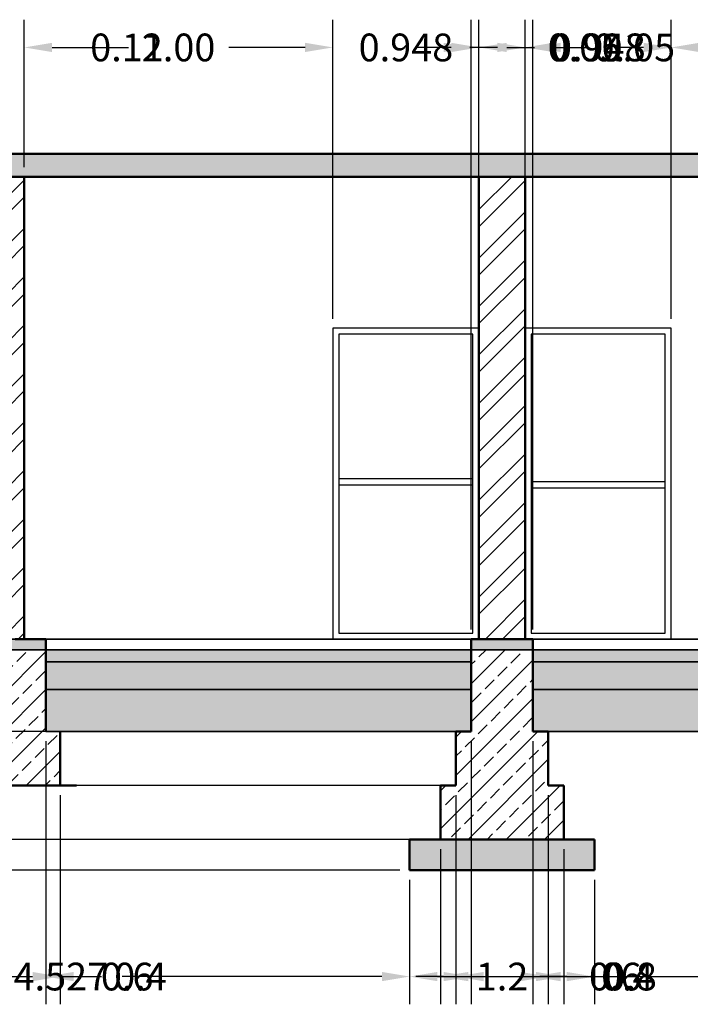
# Model space of a CAD drawing. Units: metres. Extents: x 2294.9 to 2311.3, y 1642.1 to 1648.4.
# Tile 2 of 3: x 2299.8 to 2304.1, y 1642.1 to 1648.4. Entities that reach past the tile are written whole.
import ezdxf

# ---------------------------------------------------------------- set-up
doc = ezdxf.new("R2010")
doc.units = ezdxf.units.M
for name, color, linetype, lineweight in [('A-ANNO-DIMS', 2, 'Continuous', 18), ('A-DOOR', 4, 'Continuous', 25), ('A-FLOR', 3, 'Continuous', 35), ('A-FLOR-PATT', 8, 'Continuous', 13), ('A-WALL', 7, 'Continuous', 50), ('A-WALL-PATT', 8, 'Continuous', 13), ('S-FNDN', 1, 'Continuous', 50), ('S-FNDN-PATT', 8, 'Continuous', 13), ('S-SLAB', 1, 'Continuous', 50), ('S-SLAB-PATT', 8, 'Continuous', 13)]:
    doc.layers.add(name, color=color, linetype=linetype, lineweight=lineweight)
doc.styles.get("Standard").update_dxf_attribs({"font": 'arial.ttf'})
doc.dimstyles.get("Standard").update_dxf_attribs({"dimtxt": 0.18, "dimasz": 0.18, "dimexe": 0.18, "dimexo": 0.0625, "dimgap": 0.09, "dimtad": 0, "dimtih": 1, "dimtoh": 1, "dimdec": 4, "dimzin": 0, "dimdsep": 46, "dimtxsty": 'Standard', "dimcen": 0.09, "dimadec": 0, "dimazin": 0, "dimtfac": 1, "dimtdec": 4, "dimtofl": 0, "dimtmove": 0, "dimatfit": 3, "dimfxl": 1, "dimtolj": 1, "dimtzin": 0, "dimarcsym": 0})

# ---------------------------------------------------------------- blocks, each defined once
blk = doc.blocks.new('FOOTING-PCC-PAD')
for p, q in [((1.1996, 0.1999), (-0.0004, 0.1999)), ((-0.0004, 0.1999), (-0.0004, -0.0001)), ((1.1996, -0.0001), (1.1996, 0.1999)), ((-0.0004, -0.0001), (1.1996, -0.0001))]:
    blk.add_line(p, q)
blk = doc.blocks.new('*D8')
at = {"layer": 'A-ANNO-DIMS', "color": 0, "lineweight": -2, "transparency": 16777216}
for p, q in [((2299.6895, 1647.4894), (2299.6895, 1648.4469)), ((2299.8007, 1647.4894), (2299.8007, 1648.4469)), ((2299.5095, 1648.2669), (2299.3295, 1648.2669)), ((2299.9807, 1648.2669), (2300.1607, 1648.2669))]:
    blk.add_line(p, q, dxfattribs=at)
at = {"layer": 'A-ANNO-DIMS', "color": 0, "transparency": 16777216}
for points in [[(2299.5095, 1648.2969), (2299.5095, 1648.2369), (2299.6895, 1648.2669)], [(2299.9807, 1648.2969), (2299.9807, 1648.2369), (2299.8007, 1648.2669)]]:
    blk.add_solid(points, dxfattribs=at)
at = {"layer": 'Defpoints', "color": 0, "transparency": 16777216}
for p in [(2299.8007, 1648.2669), (2299.6895, 1647.4269), (2299.8007, 1647.4269)]:
    blk.add_point(p, dxfattribs=at)
at = {"layer": 'A-ANNO-DIMS', "color": 0, "transparency": 16777216, "insert": (2300.4671, 1648.2669), "char_height": 0.18, "attachment_point": 5}
blk.add_mtext('\\A1;0.11', dxfattribs=at)
blk = doc.blocks.new('*D9')
at = {"layer": 'A-ANNO-DIMS', "color": 0, "lineweight": -2, "transparency": 16777216}
for p, q in [((2299.8007, 1647.4894), (2299.8007, 1648.4469)), ((2301.8034, 1646.5066), (2301.8034, 1648.4469)), ((2299.9807, 1648.2669), (2300.4771, 1648.2669)), ((2301.6234, 1648.2669), (2301.1271, 1648.2669))]:
    blk.add_line(p, q, dxfattribs=at)
at = {"layer": 'A-ANNO-DIMS', "color": 0, "transparency": 16777216}
for points in [[(2299.9807, 1648.2969), (2299.9807, 1648.2369), (2299.8007, 1648.2669)], [(2301.6234, 1648.2969), (2301.6234, 1648.2369), (2301.8034, 1648.2669)]]:
    blk.add_solid(points, dxfattribs=at)
at = {"layer": 'Defpoints', "color": 0, "transparency": 16777216}
for p in [(2301.8034, 1648.2669), (2299.8007, 1647.4269), (2301.8034, 1646.4441)]:
    blk.add_point(p, dxfattribs=at)
at = {"layer": 'A-ANNO-DIMS', "color": 0, "transparency": 16777216, "insert": (2300.8021, 1648.2669), "char_height": 0.18, "attachment_point": 5}
blk.add_mtext('\\A1;2.00', dxfattribs=at)
blk = doc.blocks.new('*D10')
at = {"layer": 'A-ANNO-DIMS', "color": 0, "lineweight": -2, "transparency": 16777216}
for p, q in [((2301.803421, 1646.506639), (2301.803421, 1648.446914)), ((2302.751389, 1647.489414), (2302.751389, 1648.446914)), ((2301.623421, 1648.266914), (2301.443421, 1648.266914)), ((2302.931389, 1648.266914), (2303.111389, 1648.266914))]:
    blk.add_line(p, q, dxfattribs=at)
at = {"layer": 'A-ANNO-DIMS', "color": 0, "transparency": 16777216}
for points in [[(2301.623421, 1648.296914), (2301.623421, 1648.236914), (2301.803421, 1648.266914)], [(2302.931389, 1648.296914), (2302.931389, 1648.236914), (2302.751389, 1648.266914)]]:
    blk.add_solid(points, dxfattribs=at)
at = {"layer": 'Defpoints', "color": 0, "transparency": 16777216}
for p in [(2302.751389, 1648.266914), (2302.751389, 1647.426914), (2301.803421, 1646.444139)]:
    blk.add_point(p, dxfattribs=at)
at = {"layer": 'A-ANNO-DIMS', "color": 0, "transparency": 16777216, "insert": (2302.277405, 1648.266914), "char_height": 0.18, "attachment_point": 5}
blk.add_mtext('\\A1;0.948', dxfattribs=at)
blk = doc.blocks.new('*D11')
at = {"layer": 'A-ANNO-DIMS', "color": 0, "lineweight": -2, "transparency": 16777216}
for p, q in [((2302.7514, 1647.4894), (2302.7514, 1648.4469)), ((2303.0514, 1647.4894), (2303.0514, 1648.4469)), ((2302.5714, 1648.2669), (2302.3914, 1648.2669)), ((2303.2314, 1648.2669), (2303.4114, 1648.2669))]:
    blk.add_line(p, q, dxfattribs=at)
at = {"layer": 'A-ANNO-DIMS', "color": 0, "transparency": 16777216}
for points in [[(2302.5714, 1648.2969), (2302.5714, 1648.2369), (2302.7514, 1648.2669)], [(2303.2314, 1648.2969), (2303.2314, 1648.2369), (2303.0514, 1648.2669)]]:
    blk.add_solid(points, dxfattribs=at)
at = {"layer": 'Defpoints', "color": 0, "transparency": 16777216}
for p in [(2303.0514, 1648.2669), (2302.7514, 1647.4269), (2303.0514, 1647.4269)]:
    blk.add_point(p, dxfattribs=at)
at = {"layer": 'A-ANNO-DIMS', "color": 0, "transparency": 16777216, "insert": (2303.6652, 1648.2669), "char_height": 0.18, "attachment_point": 5}
blk.add_mtext('\\A1;0.3', dxfattribs=at)
blk = doc.blocks.new('*D12')
at = {"layer": 'A-ANNO-DIMS', "color": 0, "lineweight": -2, "transparency": 16777216}
for p, q in [((2303.0514, 1647.4894), (2303.0514, 1648.4469)), ((2303.9994, 1646.5066), (2303.9994, 1648.4469)), ((2302.8714, 1648.2669), (2302.6914, 1648.2669)), ((2304.1794, 1648.2669), (2304.3594, 1648.2669))]:
    blk.add_line(p, q, dxfattribs=at)
at = {"layer": 'A-ANNO-DIMS', "color": 0, "transparency": 16777216}
for points in [[(2302.8714, 1648.2969), (2302.8714, 1648.2369), (2303.0514, 1648.2669)], [(2304.1794, 1648.2969), (2304.1794, 1648.2369), (2303.9994, 1648.2669)]]:
    blk.add_solid(points, dxfattribs=at)
at = {"layer": 'Defpoints', "color": 0, "transparency": 16777216}
for p in [(2303.9994, 1648.2669), (2303.0514, 1647.4269), (2303.9994, 1646.4441)]:
    blk.add_point(p, dxfattribs=at)
at = {"layer": 'A-ANNO-DIMS', "color": 0, "transparency": 16777216, "insert": (2303.5254, 1648.2669), "char_height": 0.18, "attachment_point": 5}
blk.add_mtext('\\A1;0.948', dxfattribs=at)
blk = doc.blocks.new('*D13')
at = {"layer": 'A-ANNO-DIMS', "color": 0, "lineweight": -2, "transparency": 16777216}
for p, q in [((2303.9994, 1646.5066), (2303.9994, 1648.4469)), ((2304.2214, 1646.5066), (2304.2214, 1648.4469)), ((2303.8194, 1648.2669), (2303.6394, 1648.2669)), ((2304.4014, 1648.2669), (2304.5814, 1648.2669))]:
    blk.add_line(p, q, dxfattribs=at)
at = {"layer": 'A-ANNO-DIMS', "color": 0, "transparency": 16777216}
for points in [[(2303.8194, 1648.2969), (2303.8194, 1648.2369), (2303.9994, 1648.2669)], [(2304.4014, 1648.2969), (2304.4014, 1648.2369), (2304.2214, 1648.2669)]]:
    blk.add_solid(points, dxfattribs=at)
at = {"layer": 'Defpoints', "color": 0, "transparency": 16777216}
for p in [(2304.2214, 1648.2669), (2303.9994, 1646.4441), (2304.2214, 1646.4441)]:
    blk.add_point(p, dxfattribs=at)
at = {"layer": 'A-ANNO-DIMS', "color": 0, "transparency": 16777216, "insert": (2304.9742, 1648.2669), "char_height": 0.18, "attachment_point": 5}
blk.add_mtext('\\A1;0.222', dxfattribs=at)
blk = doc.blocks.new('*D19')
at = {"layer": 'A-ANNO-DIMS', "color": 0, "lineweight": -2, "transparency": 16777216}
for p, q in [((2297.7746, 1642.8644), (2297.7746, 1642.0569)), ((2302.3014, 1642.8644), (2302.3014, 1642.0569)), ((2297.9546, 1642.2369), (2299.6407, 1642.2369)), ((2302.1214, 1642.2369), (2300.4353, 1642.2369))]:
    blk.add_line(p, q, dxfattribs=at)
at = {"layer": 'A-ANNO-DIMS', "color": 0, "transparency": 16777216}
for points in [[(2297.9546, 1642.2669), (2297.9546, 1642.2069), (2297.7746, 1642.2369)], [(2302.1214, 1642.2669), (2302.1214, 1642.2069), (2302.3014, 1642.2369)]]:
    blk.add_solid(points, dxfattribs=at)
at = {"layer": 'Defpoints', "color": 0, "transparency": 16777216}
for p in [(2297.7746, 1642.9269), (2302.3014, 1642.9269), (2302.3014, 1642.2369)]:
    blk.add_point(p, dxfattribs=at)
at = {"layer": 'A-ANNO-DIMS', "color": 0, "transparency": 16777216, "insert": (2300.038, 1642.2369), "char_height": 0.18, "attachment_point": 5}
blk.add_mtext('\\A1;4.527', dxfattribs=at)
blk = doc.blocks.new('*D20')
at = {"layer": 'A-ANNO-DIMS', "color": 0, "lineweight": -2, "transparency": 16777216}
for p, q in [((2302.3014, 1642.8644), (2302.3014, 1642.0569)), ((2303.5014, 1642.8644), (2303.5014, 1642.0569)), ((2302.4814, 1642.2369), (2302.6569, 1642.2369)), ((2303.3214, 1642.2369), (2303.1459, 1642.2369))]:
    blk.add_line(p, q, dxfattribs=at)
at = {"layer": 'A-ANNO-DIMS', "color": 0, "transparency": 16777216}
for points in [[(2302.4814, 1642.2669), (2302.4814, 1642.2069), (2302.3014, 1642.2369)], [(2303.3214, 1642.2669), (2303.3214, 1642.2069), (2303.5014, 1642.2369)]]:
    blk.add_solid(points, dxfattribs=at)
at = {"layer": 'Defpoints', "color": 0, "transparency": 16777216}
for p in [(2302.3014, 1642.9269), (2303.5014, 1642.9269), (2303.5014, 1642.2369)]:
    blk.add_point(p, dxfattribs=at)
at = {"layer": 'A-ANNO-DIMS', "color": 0, "transparency": 16777216, "insert": (2302.9014, 1642.2369), "char_height": 0.18, "attachment_point": 5}
blk.add_mtext('\\A1;1.2', dxfattribs=at)
blk = doc.blocks.new('*D21')
at = {"layer": 'A-ANNO-DIMS', "color": 0, "lineweight": -2, "transparency": 16777216}
for p, q in [((2302.3014, 1642.8644), (2302.3014, 1642.0569)), ((2308.0253, 1642.8644), (2308.0253, 1642.0569)), ((2302.4814, 1642.2369), (2304.77, 1642.2369)), ((2307.8453, 1642.2369), (2305.5567, 1642.2369))]:
    blk.add_line(p, q, dxfattribs=at)
at = {"layer": 'A-ANNO-DIMS', "color": 0, "transparency": 16777216}
for points in [[(2302.4814, 1642.2669), (2302.4814, 1642.2069), (2302.3014, 1642.2369)], [(2307.8453, 1642.2669), (2307.8453, 1642.2069), (2308.0253, 1642.2369)]]:
    blk.add_solid(points, dxfattribs=at)
at = {"layer": 'Defpoints', "color": 0, "transparency": 16777216}
for p in [(2302.3014, 1642.9269), (2308.0253, 1642.9269), (2308.0253, 1642.2369)]:
    blk.add_point(p, dxfattribs=at)
at = {"layer": 'A-ANNO-DIMS', "color": 0, "transparency": 16777216, "insert": (2305.1633, 1642.2369), "char_height": 0.18, "attachment_point": 5}
blk.add_mtext('\\A1;5.724', dxfattribs=at)
blk = doc.blocks.new('*D23')
at = {"layer": 'A-ANNO-DIMS', "color": 0, "lineweight": -2, "transparency": 16777216}
for p, q in [((2299.5412, 1643.7644), (2299.5412, 1642.0569)), ((2299.9412, 1643.7644), (2299.9412, 1642.0569)), ((2299.3612, 1642.2369), (2299.1812, 1642.2369)), ((2300.1212, 1642.2369), (2300.3012, 1642.2369))]:
    blk.add_line(p, q, dxfattribs=at)
at = {"layer": 'A-ANNO-DIMS', "color": 0, "transparency": 16777216}
for points in [[(2299.3612, 1642.2669), (2299.3612, 1642.2069), (2299.5412, 1642.2369)], [(2300.1212, 1642.2669), (2300.1212, 1642.2069), (2299.9412, 1642.2369)]]:
    blk.add_solid(points, dxfattribs=at)
at = {"layer": 'Defpoints', "color": 0, "transparency": 16777216}
for p in [(2299.5412, 1643.8269), (2299.9412, 1643.8269), (2299.9412, 1642.2369)]:
    blk.add_point(p, dxfattribs=at)
at = {"layer": 'A-ANNO-DIMS', "color": 0, "transparency": 16777216, "insert": (2300.5547, 1642.2369), "char_height": 0.18, "attachment_point": 5}
blk.add_mtext('\\A1;0.4', dxfattribs=at)
blk = doc.blocks.new('*D24')
at = {"layer": 'A-ANNO-DIMS', "color": 0, "lineweight": -2, "transparency": 16777216}
for p, q in [((2299.4343, 1643.4144), (2299.4343, 1642.0569)), ((2300.0343, 1643.4144), (2300.0343, 1642.0569)), ((2299.6143, 1642.2369), (2299.8543, 1642.2369)), ((2300.0343, 1642.2369), (2300.2143, 1642.2369))]:
    blk.add_line(p, q, dxfattribs=at)
at = {"layer": 'A-ANNO-DIMS', "color": 0, "transparency": 16777216}
for points in [[(2299.6143, 1642.2669), (2299.6143, 1642.2069), (2299.4343, 1642.2369)], [(2299.8543, 1642.2669), (2299.8543, 1642.2069), (2300.0343, 1642.2369)]]:
    blk.add_solid(points, dxfattribs=at)
at = {"layer": 'Defpoints', "color": 0, "transparency": 16777216}
for p in [(2299.4343, 1643.4769), (2300.0343, 1643.4769), (2300.0343, 1642.2369)]:
    blk.add_point(p, dxfattribs=at)
at = {"layer": 'A-ANNO-DIMS', "color": 0, "transparency": 16777216, "insert": (2300.4681, 1642.2369), "char_height": 0.18, "attachment_point": 5}
blk.add_mtext('\\A1;0.6', dxfattribs=at)
blk = doc.blocks.new('*D25')
at = {"layer": 'A-ANNO-DIMS', "color": 0, "lineweight": -2, "transparency": 16777216}
for p, q in [((2302.7014, 1644.4894), (2302.7014, 1648.4469)), ((2302.7514, 1644.4894), (2302.7514, 1648.4469)), ((2302.5214, 1648.2669), (2302.3414, 1648.2669)), ((2302.9314, 1648.2669), (2303.1114, 1648.2669))]:
    blk.add_line(p, q, dxfattribs=at)
at = {"layer": 'A-ANNO-DIMS', "color": 0, "transparency": 16777216}
for points in [[(2302.5214, 1648.2969), (2302.5214, 1648.2369), (2302.7014, 1648.2669)], [(2302.9314, 1648.2969), (2302.9314, 1648.2369), (2302.7514, 1648.2669)]]:
    blk.add_solid(points, dxfattribs=at)
at = {"layer": 'Defpoints', "color": 0, "transparency": 16777216}
for p in [(2302.7514, 1648.2669), (2302.7014, 1644.4269), (2302.7514, 1644.4269)]:
    blk.add_point(p, dxfattribs=at)
at = {"layer": 'A-ANNO-DIMS', "color": 0, "transparency": 16777216, "insert": (2303.4358, 1648.2669), "char_height": 0.18, "attachment_point": 5}
blk.add_mtext('\\A1;0.05', dxfattribs=at)
blk = doc.blocks.new('*D26')
at = {"layer": 'A-ANNO-DIMS', "color": 0, "lineweight": -2, "transparency": 16777216}
for p, q in [((2302.7514, 1644.4894), (2302.7514, 1648.4469)), ((2303.0514, 1644.4894), (2303.0514, 1648.4469)), ((2302.5714, 1648.2669), (2302.3914, 1648.2669)), ((2303.2314, 1648.2669), (2303.4114, 1648.2669))]:
    blk.add_line(p, q, dxfattribs=at)
at = {"layer": 'A-ANNO-DIMS', "color": 0, "transparency": 16777216}
for points in [[(2302.5714, 1648.2969), (2302.5714, 1648.2369), (2302.7514, 1648.2669)], [(2303.2314, 1648.2969), (2303.2314, 1648.2369), (2303.0514, 1648.2669)]]:
    blk.add_solid(points, dxfattribs=at)
at = {"layer": 'Defpoints', "color": 0, "transparency": 16777216}
for p in [(2303.0514, 1648.2669), (2302.7514, 1644.4269), (2303.0514, 1644.4269)]:
    blk.add_point(p, dxfattribs=at)
at = {"layer": 'A-ANNO-DIMS', "color": 0, "transparency": 16777216, "insert": (2303.6652, 1648.2669), "char_height": 0.18, "attachment_point": 5}
blk.add_mtext('\\A1;0.3', dxfattribs=at)
blk = doc.blocks.new('*D27')
at = {"layer": 'A-ANNO-DIMS', "color": 0, "lineweight": -2, "transparency": 16777216}
for p, q in [((2303.0514, 1644.4894), (2303.0514, 1648.4469)), ((2303.1014, 1644.4894), (2303.1014, 1648.4469)), ((2302.8714, 1648.2669), (2302.6914, 1648.2669)), ((2303.2814, 1648.2669), (2303.4614, 1648.2669))]:
    blk.add_line(p, q, dxfattribs=at)
at = {"layer": 'A-ANNO-DIMS', "color": 0, "transparency": 16777216}
for points in [[(2302.8714, 1648.2969), (2302.8714, 1648.2369), (2303.0514, 1648.2669)], [(2303.2814, 1648.2969), (2303.2814, 1648.2369), (2303.1014, 1648.2669)]]:
    blk.add_solid(points, dxfattribs=at)
at = {"layer": 'Defpoints', "color": 0, "transparency": 16777216}
for p in [(2303.1014, 1648.2669), (2303.0514, 1644.4269), (2303.1014, 1644.4269)]:
    blk.add_point(p, dxfattribs=at)
at = {"layer": 'A-ANNO-DIMS', "color": 0, "transparency": 16777216, "insert": (2303.7858, 1648.2669), "char_height": 0.18, "attachment_point": 5}
blk.add_mtext('\\A1;0.05', dxfattribs=at)
blk = doc.blocks.new('*D28')
at = {"layer": 'A-ANNO-DIMS', "color": 0, "lineweight": -2, "transparency": 16777216}
for p, q in [((2302.7014, 1643.7644), (2302.7014, 1642.0569)), ((2303.1014, 1643.7644), (2303.1014, 1642.0569)), ((2302.5214, 1642.2369), (2302.3414, 1642.2369)), ((2303.2814, 1642.2369), (2303.4614, 1642.2369))]:
    blk.add_line(p, q, dxfattribs=at)
at = {"layer": 'A-ANNO-DIMS', "color": 0, "transparency": 16777216}
for points in [[(2302.5214, 1642.2669), (2302.5214, 1642.2069), (2302.7014, 1642.2369)], [(2303.2814, 1642.2669), (2303.2814, 1642.2069), (2303.1014, 1642.2369)]]:
    blk.add_solid(points, dxfattribs=at)
at = {"layer": 'Defpoints', "color": 0, "transparency": 16777216}
for p in [(2302.7014, 1643.8269), (2303.1014, 1643.8269), (2303.1014, 1642.2369)]:
    blk.add_point(p, dxfattribs=at)
at = {"layer": 'A-ANNO-DIMS', "color": 0, "transparency": 16777216, "insert": (2303.7149, 1642.2369), "char_height": 0.18, "attachment_point": 5}
blk.add_mtext('\\A1;0.4', dxfattribs=at)
blk = doc.blocks.new('*D29')
at = {"layer": 'A-ANNO-DIMS', "color": 0, "lineweight": -2, "transparency": 16777216}
for p, q in [((2302.6014, 1643.4144), (2302.6014, 1642.0569)), ((2303.2014, 1643.4144), (2303.2014, 1642.0569)), ((2302.7814, 1642.2369), (2303.0214, 1642.2369)), ((2303.2014, 1642.2369), (2303.3814, 1642.2369))]:
    blk.add_line(p, q, dxfattribs=at)
at = {"layer": 'A-ANNO-DIMS', "color": 0, "transparency": 16777216}
for points in [[(2302.7814, 1642.2669), (2302.7814, 1642.2069), (2302.6014, 1642.2369)], [(2303.0214, 1642.2669), (2303.0214, 1642.2069), (2303.2014, 1642.2369)]]:
    blk.add_solid(points, dxfattribs=at)
at = {"layer": 'Defpoints', "color": 0, "transparency": 16777216}
for p in [(2302.6014, 1643.4769), (2303.2014, 1643.4769), (2303.2014, 1642.2369)]:
    blk.add_point(p, dxfattribs=at)
at = {"layer": 'A-ANNO-DIMS', "color": 0, "transparency": 16777216, "insert": (2303.6352, 1642.2369), "char_height": 0.18, "attachment_point": 5}
blk.add_mtext('\\A1;0.6', dxfattribs=at)
blk = doc.blocks.new('*D30')
at = {"layer": 'A-ANNO-DIMS', "color": 0, "lineweight": -2, "transparency": 16777216}
for p, q in [((2302.5014, 1643.0644), (2302.5014, 1642.0569)), ((2303.3014, 1643.0644), (2303.3014, 1642.0569)), ((2302.6814, 1642.2369), (2303.1214, 1642.2369)), ((2303.3014, 1642.2369), (2303.4814, 1642.2369))]:
    blk.add_line(p, q, dxfattribs=at)
at = {"layer": 'A-ANNO-DIMS', "color": 0, "transparency": 16777216}
for points in [[(2302.6814, 1642.2669), (2302.6814, 1642.2069), (2302.5014, 1642.2369)], [(2303.1214, 1642.2669), (2303.1214, 1642.2069), (2303.3014, 1642.2369)]]:
    blk.add_solid(points, dxfattribs=at)
at = {"layer": 'Defpoints', "color": 0, "transparency": 16777216}
for p in [(2302.5014, 1643.1269), (2303.3014, 1643.1269), (2303.3014, 1642.2369)]:
    blk.add_point(p, dxfattribs=at)
at = {"layer": 'A-ANNO-DIMS', "color": 0, "transparency": 16777216, "insert": (2303.7354, 1642.2369), "char_height": 0.18, "attachment_point": 5}
blk.add_mtext('\\A1;0.8', dxfattribs=at)
blk = doc.blocks.new('*D31')
at = {"layer": 'A-ANNO-DIMS', "color": 0, "lineweight": -2, "transparency": 16777216}
for p, q in [((2295.6583, 1644.0069), (2295.6583, 1644.1869)), ((2302.5389, 1643.8269), (2295.4783, 1643.8269)), ((2302.5389, 1643.4769), (2295.4783, 1643.4769)), ((2295.6583, 1643.2969), (2295.6583, 1643.1169)), ((2295.6583, 1643.1169), (2295.4783, 1643.1169))]:
    blk.add_line(p, q, dxfattribs=at)
at = {"layer": 'A-ANNO-DIMS', "color": 0, "transparency": 16777216}
for points in [[(2295.6283, 1644.0069), (2295.6883, 1644.0069), (2295.6583, 1643.8269)], [(2295.6283, 1643.2969), (2295.6883, 1643.2969), (2295.6583, 1643.4769)]]:
    blk.add_solid(points, dxfattribs=at)
at = {"layer": 'Defpoints', "color": 0, "transparency": 16777216}
for p in [(2302.6014, 1643.8269), (2295.6583, 1643.4769), (2302.6014, 1643.4769)]:
    blk.add_point(p, dxfattribs=at)
at = {"layer": 'A-ANNO-DIMS', "color": 0, "transparency": 16777216, "insert": (2295.1539, 1643.1169), "char_height": 0.18, "attachment_point": 5}
blk.add_mtext('\\A1;0.35', dxfattribs=at)
blk = doc.blocks.new('*D32')
at = {"layer": 'A-ANNO-DIMS', "color": 0, "lineweight": -2, "transparency": 16777216}
for p, q in [((2295.6583, 1643.6569), (2295.6583, 1643.8369)), ((2302.4389, 1643.4769), (2295.4783, 1643.4769)), ((2302.4389, 1643.1269), (2295.4783, 1643.1269)), ((2295.6583, 1642.9469), (2295.6583, 1642.7669)), ((2295.6583, 1642.7669), (2295.4783, 1642.7669))]:
    blk.add_line(p, q, dxfattribs=at)
at = {"layer": 'A-ANNO-DIMS', "color": 0, "transparency": 16777216}
for points in [[(2295.6283, 1643.6569), (2295.6883, 1643.6569), (2295.6583, 1643.4769)], [(2295.6283, 1642.9469), (2295.6883, 1642.9469), (2295.6583, 1643.1269)]]:
    blk.add_solid(points, dxfattribs=at)
at = {"layer": 'Defpoints', "color": 0, "transparency": 16777216}
for p in [(2302.5014, 1643.4769), (2295.6583, 1643.1269), (2302.5014, 1643.1269)]:
    blk.add_point(p, dxfattribs=at)
at = {"layer": 'A-ANNO-DIMS', "color": 0, "transparency": 16777216, "insert": (2295.1539, 1642.7669), "char_height": 0.18, "attachment_point": 5}
blk.add_mtext('\\A1;0.35', dxfattribs=at)
blk = doc.blocks.new('*D33')
at = {"layer": 'A-ANNO-DIMS', "color": 0, "lineweight": -2, "transparency": 16777216}
for p, q in [((2295.6583, 1643.3069), (2295.6583, 1643.4869)), ((2302.2389, 1643.1269), (2295.4783, 1643.1269)), ((2302.2389, 1642.9269), (2295.4783, 1642.9269)), ((2295.6583, 1642.7469), (2295.6583, 1642.5669)), ((2295.6583, 1642.5669), (2295.4783, 1642.5669))]:
    blk.add_line(p, q, dxfattribs=at)
at = {"layer": 'A-ANNO-DIMS', "color": 0, "transparency": 16777216}
for points in [[(2295.6283, 1643.3069), (2295.6883, 1643.3069), (2295.6583, 1643.1269)], [(2295.6283, 1642.7469), (2295.6883, 1642.7469), (2295.6583, 1642.9269)]]:
    blk.add_solid(points, dxfattribs=at)
at = {"layer": 'Defpoints', "color": 0, "transparency": 16777216}
for p in [(2302.3014, 1643.1269), (2295.6583, 1642.9269), (2302.3014, 1642.9269)]:
    blk.add_point(p, dxfattribs=at)
at = {"layer": 'A-ANNO-DIMS', "color": 0, "transparency": 16777216, "insert": (2295.2254, 1642.5669), "char_height": 0.18, "attachment_point": 5}
blk.add_mtext('\\A1;0.2', dxfattribs=at)
blk = doc.blocks.new('*D34')
at = {"layer": 'A-ANNO-DIMS', "color": 0, "lineweight": -2, "transparency": 16777216}
for p, q in [((2302.6389, 1644.4269), (2295.4783, 1644.4269)), ((2295.6583, 1644.2469), (2295.6583, 1644.0069)), ((2302.6389, 1643.8269), (2295.4783, 1643.8269)), ((2295.6583, 1643.8269), (2295.6583, 1643.6469)), ((2295.6583, 1643.6469), (2295.4783, 1643.6469))]:
    blk.add_line(p, q, dxfattribs=at)
at = {"layer": 'A-ANNO-DIMS', "color": 0, "transparency": 16777216}
for points in [[(2295.6283, 1644.2469), (2295.6883, 1644.2469), (2295.6583, 1644.4269)], [(2295.6283, 1644.0069), (2295.6883, 1644.0069), (2295.6583, 1643.8269)]]:
    blk.add_solid(points, dxfattribs=at)
at = {"layer": 'Defpoints', "color": 0, "transparency": 16777216}
for p in [(2302.7014, 1644.4269), (2295.6583, 1643.8269), (2302.7014, 1643.8269)]:
    blk.add_point(p, dxfattribs=at)
at = {"layer": 'A-ANNO-DIMS', "color": 0, "transparency": 16777216, "insert": (2295.2245, 1643.6469), "char_height": 0.18, "attachment_point": 5}
blk.add_mtext('\\A1;0.6', dxfattribs=at)
blk = doc.blocks.new('*D35')
at = {"layer": 'A-ANNO-DIMS', "color": 0, "lineweight": -2, "transparency": 16777216}
for p, q in [((2310.5137, 1644.4597), (2310.5137, 1644.6397)), ((2303.1639, 1644.2797), (2310.6937, 1644.2797)), ((2303.1639, 1644.1004), (2310.6937, 1644.1004)), ((2310.5137, 1643.9204), (2310.5137, 1643.7404)), ((2310.5137, 1643.7404), (2310.3337, 1643.7404))]:
    blk.add_line(p, q, dxfattribs=at)
at = {"layer": 'A-ANNO-DIMS', "color": 0, "transparency": 16777216}
for points in [[(2310.4837, 1644.4597), (2310.5437, 1644.4597), (2310.5137, 1644.2797)], [(2310.4837, 1643.9204), (2310.5437, 1643.9204), (2310.5137, 1644.1004)]]:
    blk.add_solid(points, dxfattribs=at)
at = {"layer": 'Defpoints', "color": 0, "transparency": 16777216}
for p in [(2303.1014, 1644.2797), (2303.1014, 1644.1004), (2310.5137, 1644.1004)]:
    blk.add_point(p, dxfattribs=at)
at = {"layer": 'A-ANNO-DIMS', "color": 0, "transparency": 16777216, "insert": (2310.0097, 1643.7404), "char_height": 0.18, "attachment_point": 5}
blk.add_mtext('\\A1;0.18', dxfattribs=at)
blk = doc.blocks.new('*D36')
at = {"layer": 'A-ANNO-DIMS', "color": 0, "lineweight": -2, "transparency": 16777216}
for p, q in [((2310.5137, 1644.2804), (2310.5137, 1644.4604)), ((2303.1639, 1644.1004), (2310.6937, 1644.1004)), ((2303.1639, 1643.8269), (2310.6937, 1643.8269)), ((2310.5137, 1643.6469), (2310.5137, 1643.4669)), ((2310.5137, 1643.4669), (2310.3337, 1643.4669))]:
    blk.add_line(p, q, dxfattribs=at)
at = {"layer": 'A-ANNO-DIMS', "color": 0, "transparency": 16777216}
for points in [[(2310.4837, 1644.2804), (2310.5437, 1644.2804), (2310.5137, 1644.1004)], [(2310.4837, 1643.6469), (2310.5437, 1643.6469), (2310.5137, 1643.8269)]]:
    blk.add_solid(points, dxfattribs=at)
at = {"layer": 'Defpoints', "color": 0, "transparency": 16777216}
for p in [(2303.1014, 1644.1004), (2303.1014, 1643.8269), (2310.5137, 1643.8269)]:
    blk.add_point(p, dxfattribs=at)
at = {"layer": 'A-ANNO-DIMS', "color": 0, "transparency": 16777216, "insert": (2310.0099, 1643.4669), "char_height": 0.18, "attachment_point": 5}
blk.add_mtext('\\A1;0.27', dxfattribs=at)

msp = doc.modelspace()

# ---------------------------------------------------------------- hatches: boundary and pattern name
at = {"layer": 'A-FLOR-PATT'}
h = msp.add_hatch(dxfattribs=at)
h.set_pattern_fill('JIS_STN_2.5', color=256, scale=0.07)
h.paths.add_polyline_path([(2297.3746, 1644.3583), (2296.9746, 1644.3583), (2296.9746, 1644.3269), (2296.9746, 1643.8269), (2296.8746, 1643.8269), (2296.8746, 1643.4769), (2296.7746, 1643.4769), (2296.7746, 1643.1269), (2297.5746, 1643.1269), (2297.5746, 1643.4769), (2297.4746, 1643.4769), (2297.4746, 1643.8269), (2297.3746, 1643.8269)])
h.paths.add_polyline_path([(2300.0343, 1643.8269), (2299.9412, 1643.8269), (2299.9412, 1644.3583), (2299.5412, 1644.3583), (2299.5412, 1643.8269), (2299.4343, 1643.8269), (2299.4343, 1643.4769), (2299.6329, 1643.4769), (2299.6744, 1643.5859), (2299.6809, 1643.3504), (2299.7223, 1643.4769), (2300.0343, 1643.4769)])
h.paths.add_polyline_path([(2303.2014, 1643.8269), (2303.1014, 1643.8269), (2303.1014, 1644.3583), (2302.7014, 1644.3583), (2302.7014, 1643.8269), (2302.6014, 1643.8269), (2302.6014, 1643.4769), (2302.5014, 1643.4769), (2302.5014, 1643.1269), (2303.3014, 1643.1269), (2303.3014, 1643.4769), (2303.2014, 1643.4769)])
h.paths.add_polyline_path([(2308.9253, 1643.8269), (2308.8253, 1643.8269), (2308.8253, 1644.3583), (2308.4253, 1644.3583), (2308.4253, 1643.8269), (2308.3253, 1643.8269), (2308.3253, 1643.4769), (2308.2253, 1643.4769), (2308.2253, 1643.1269), (2309.0253, 1643.1269), (2309.0253, 1643.4769), (2308.9253, 1643.4769)])
h = msp.add_hatch(dxfattribs=at)
h.set_pattern_fill('AR-SAND', color=256, scale=0.001)
h.paths.add_polyline_path([(2302.7014, 1644.3583), (2299.9412, 1644.3583), (2299.9412, 1644.2797), (2302.7014, 1644.2797)])
h.paths.add_polyline_path([(2308.4253, 1644.3583), (2303.1014, 1644.3583), (2303.1014, 1644.2797), (2308.4253, 1644.2797)])
h = msp.add_hatch(dxfattribs=at)
h.set_pattern_fill('AR-CONC', color=256, scale=0.002)
h.paths.add_polyline_path([(2299.5412, 1644.2797), (2297.3746, 1644.2797), (2297.3746, 1644.1004), (2299.5412, 1644.1004)])
h.paths.add_polyline_path([(2302.7014, 1644.2797), (2299.9412, 1644.2797), (2299.9412, 1644.1004), (2302.7014, 1644.1004)])
h.paths.add_polyline_path([(2308.4253, 1644.2797), (2303.1014, 1644.2797), (2303.1014, 1644.1004), (2308.4253, 1644.1004)])
h = msp.add_hatch(dxfattribs=at)
h.set_pattern_fill('GRAVEL', color=256, scale=0.01)
h.set_pattern_definition([(228.0127875, (0.18288, 0.254), (-2.03200000016, -2.28599999986), [0.034172144, -3.383048364]), (184.969741, (0.16002, 0.2286), (3.047999998794, 0.25400001447), [0.058640472, -5.80540489]), (132.5104471, (0.1016, 0.22352), (2.54000000107, -2.793999999025), [0.041348152, -4.09347228]), (267.273689, (0.00254, 0.16002), (0.25400000053, 5.079999999973), [0.053400452, -5.286643743]), (292.8336542, (0, 0.10668), (-1.270000000106, 3.047999999956), [0.05236337, -5.183980775]), (357.273689, (0.02032, 0.05842), (-5.079999999973, 0.25400000053), [0.053400452, -5.286643743]), (37.69424047, (0.07366, 0.05588), (-3.301999999854, -2.54000000019), [0.070619366, -6.991311531]), (72.25532837, (0.12954, 0.09906), (1.778000000478, 5.587999999848), [0.066671952, -6.60052566]), (121.4295656, (0.14986, 0.16256), (-2.03200000029, 3.301999999823), [0.0535813, -5.30455457]), (175.2363583, (0.12192, 0.20828), (2.79399999996, -0.25400000044), [0.061171328, -2.997393695]), (222.3974378, (0.06096, 0.21336), (-3.047999999902, -2.794000000106), [0.079107792, -7.831677251]), (138.8140748, (0.254, 0.15748), (-1.7779999999, 1.52400000012), [0.027000454, -2.673056582]), (171.4692344, (0.23368, 0.17526), (3.30200000009, -0.507999999424), [0.051368198, -5.0854639]), (225, (0.18288, 0.18288), (0, -0.254), [0.035920934, -0.32328931]), (203.1985905, (0.1651, 0.21336), (1.27000000003, 0.5079999999), [0.019344132, -1.915062237]), (291.8014095, (0.14732, 0.20574), (-0.25400000005, 0.762), [0.027356562, -1.3404753]), (30.9637565, (0.15748, 0.18034), (0.762, 0.508), [0.044431966, -1.436629815]), (161.5650512, (0.19558, 0.2032), (0.508, -0.254), [0.032128714, -0.771089812]), (16.38954033, (0, 0.20574), (2.54, 0.762), [0.0450088, -4.455882667]), (70.34617594, (0.04318, 0.21844), (-1.01600000009, -2.79399999997), [0.037759894, -3.738221568]), (293.1985905, (0.19558, 0.254), (-0.5079999999, 1.27000000004), [0.03868801, -1.89571836]), (343.61045967, (0.21082, 0.21844), (-2.54000000005, 0.76199999982), [0.0450088, -4.455882667]), (339.4439548, (0, 0.04826), (-1.27, 0.508), [0.04340352, -2.126773431]), (294.7751406, (0.04064, 0.03302), (-1.27000000151, 2.79399999931), [0.036367212, -3.600359338]), (66.8014095, (0.19812, 0), (0.50799999992, 1.27000000003), [0.03868801, -1.89571836]), (17.35402464, (0.21336, 0.03556), (-3.301999999934, -1.01600000021), [0.042578274, -4.215237598]), (69.4439548, (0.07366, 0), (-0.508, -1.27), [0.02170176, -2.148475191]), (101.3099325, (0.18288, 0), (-0.254, 1.016), [0.01295146, -1.282199496]), (165.9637565, (0.18034, 0.0127), (0.762, -0.254), [0.05236337, -0.99490546]), (186.00900596, (0.12954, 0.0254), (2.539999999987, 0.25400000013), [0.0485267, -4.804136486]), (303.6900675, (0.15748, 0.15748), (-0.254, 0.508), [0.036632388, -0.879177636]), (353.1572266, (0.1778, 0.127), (4.318000000027, -0.507999999774), [0.063955676, -6.331600907]), (60.9453959, (0.2413, 0.11938), (-1.01600000003, -1.77799999998), [0.026150824, -2.588939232]), (90, (0.254, 0.14224), (-0.254, 0.254), [0.01524, -0.23876]), (120.25643716, (0.12446, 0.03302), (1.01599999988, -1.77800000007), [0.035286696, -3.493394077]), (48.0127875, (0.10668, 0.0635), (2.03200000017, 2.28599999985), [0.068344288, -3.34887622]), (0, (0.1524, 0.1143), (0.254, 0.254), [0.06604, -0.18796]), (325.3048465, (0.21844, 0.1143), (2.54000000096, -1.77799999863), [0.040160956, -3.975931672]), (254.0546041, (0.25146, 0.09144), (-0.254, -1.016), [0.036982908, -1.812165004]), (207.64597536, (0.2413, 0.05588), (-4.826000000177, -2.539999999663), [0.06021451, -5.961246442]), (175.42607874, (0.18796, 0.02794), (-3.302, 0.254), [0.063702946, -6.306584646])])
h.paths.add_polyline_path([(2299.5412, 1644.1004), (2297.3746, 1644.1004), (2297.3746, 1643.8269), (2297.4746, 1643.8269), (2299.5412, 1643.8269)])
h.paths.add_polyline_path([(2302.7014, 1644.1004), (2299.9412, 1644.1004), (2299.9412, 1643.8269), (2302.7014, 1643.8269)])
h.paths.add_polyline_path([(2308.4253, 1644.1004), (2303.1014, 1644.1004), (2303.1014, 1643.8269), (2308.4253, 1643.8269)])
at = {"layer": 'A-WALL-PATT'}
h = msp.add_hatch(dxfattribs=at)
h.set_pattern_fill('STEEL', color=256, scale=0.07)
h.set_pattern_definition([(45, (0, 0), (-0.157154482, 0.157154482), []), (45, (0, 0.11113), (-0.157154482, 0.157154482), [])])
h.paths.add_polyline_path([(2297.3246, 1646.4471), (2297.0246, 1646.4471), (2297.0246, 1644.4269), (2297.3246, 1644.4269)])
h.paths.add_polyline_path([(2297.3246, 1647.4269), (2297.1746, 1647.4269), (2297.0246, 1647.4269), (2297.0246, 1647.0586), (2297.3246, 1647.0586)])
h.paths.add_polyline_path([(2299.8007, 1647.4269), (2299.6895, 1647.4269), (2299.6895, 1644.4269), (2299.7412, 1644.4269), (2299.8007, 1644.4269)])
h.paths.add_polyline_path([(2303.0514, 1646.4441), (2303.0514, 1647.4269), (2302.7514, 1647.4269), (2302.7514, 1644.4269), (2303.0514, 1644.4269)])
at = {"layer": 'S-FNDN-PATT'}
h = msp.add_hatch(dxfattribs=at)
h.set_pattern_fill('AR-CONC', color=256, scale=0.001)
h.paths.add_polyline_path([(2297.7746, 1643.1269), (2296.5746, 1643.1269), (2296.5746, 1642.9269), (2297.7746, 1642.9269)])
h.paths.add_polyline_path([(2303.5014, 1643.1269), (2302.3014, 1643.1269), (2302.3014, 1642.9269), (2303.5014, 1642.9269)])
h.paths.add_polyline_path([(2309.2253, 1643.1269), (2308.0253, 1643.1269), (2308.0253, 1642.9269), (2309.2253, 1642.9269)])
h.paths.add_polyline_path([(2297.3746, 1644.4269), (2297.3246, 1644.4269), (2297.0246, 1644.4269), (2296.9746, 1644.4269), (2296.9746, 1644.3583), (2297.3746, 1644.3583)])
h.paths.add_polyline_path([(2299.9412, 1644.4269), (2299.7412, 1644.4269), (2299.5412, 1644.4269), (2299.5412, 1644.3583), (2299.9412, 1644.3583)])
h.paths.add_polyline_path([(2303.1014, 1644.4269), (2303.0514, 1644.4269), (2302.7514, 1644.4269), (2302.7014, 1644.4269), (2302.7014, 1644.3583), (2303.1014, 1644.3583)])
h.paths.add_polyline_path([(2308.8253, 1644.4269), (2308.7753, 1644.4269), (2308.4753, 1644.4269), (2308.4253, 1644.4269), (2308.4253, 1644.3583), (2308.8253, 1644.3583)])
at = {"layer": 'S-SLAB-PATT'}
h = msp.add_hatch(dxfattribs=at)
h.set_pattern_fill('AR-CONC', color=256, scale=0.002)
h.paths.add_polyline_path([(2309.2101, 1647.5769), (2296.8101, 1647.5769), (2296.8101, 1647.4269), (2297.1746, 1647.4269), (2308.6282, 1647.4269), (2309.2101, 1647.4269)])

# ---------------------------------------------------------------- linework, layer by layer
at = {"layer": 'A-DOOR'}
for p, q in [((2301.8423, 1645.4696), (2302.7125, 1645.4696)), ((2301.8423, 1645.4273), (2302.7125, 1645.4273)), ((2303.0903, 1645.4502), (2303.9605, 1645.4502)), ((2303.0903, 1645.4079), (2303.9605, 1645.4079))]:
    msp.add_line(p, q, dxfattribs=at)
for points in [[(2302.7514, 1646.4441), (2301.8034, 1646.4441), (2301.8034, 1644.4269), (2302.7514, 1644.4269)], [(2302.7125, 1646.4052), (2301.8423, 1646.4052), (2301.8423, 1644.4658), (2302.7125, 1644.4658)], [(2303.9994, 1646.4441), (2303.0514, 1646.4441), (2303.0514, 1644.4269), (2303.9994, 1644.4269)], [(2303.9605, 1646.4052), (2303.0903, 1646.4052), (2303.0903, 1644.4658), (2303.9605, 1644.4658)]]:
    msp.add_lwpolyline(points, close=True, dxfattribs=at)
at = {"layer": 'A-FLOR'}
for p, q in [((2297.3746, 1644.4269), (2302.7514, 1644.4269)), ((2303.0514, 1644.4269), (2308.4253, 1644.4269)), ((2296.9746, 1644.3583), (2308.8253, 1644.3583)), ((2299.9412, 1644.2797), (2302.7014, 1644.2797)), ((2303.1014, 1644.2797), (2308.4253, 1644.2797)), ((2299.9412, 1644.1004), (2302.7014, 1644.1004)), ((2303.1014, 1644.1004), (2308.4253, 1644.1004)), ((2299.9412, 1643.8269), (2302.7014, 1643.8269)), ((2303.1014, 1643.8269), (2308.4253, 1643.8269))]:
    msp.add_line(p, q, dxfattribs=at)
at = {"layer": 'A-WALL'}
for p, q in [((2299.8007, 1647.4269), (2299.8007, 1644.4269)), ((2302.7514, 1644.4269), (2302.7514, 1647.4269)), ((2303.0514, 1644.4269), (2303.0514, 1647.4269)), ((2302.7514, 1644.4269), (2303.0514, 1644.4269))]:
    msp.add_line(p, q, dxfattribs=at)
at = {"layer": 'S-FNDN'}
for p, q in [((2299.7412, 1644.4269), (2299.9412, 1644.4269)), ((2299.9412, 1644.4269), (2299.9412, 1643.8269)), ((2302.7014, 1643.8269), (2302.7014, 1644.4269)), ((2302.7014, 1644.4269), (2302.7514, 1644.4269)), ((2303.0514, 1644.4269), (2303.1014, 1644.4269)), ((2303.1014, 1644.4269), (2303.1014, 1643.8269)), ((2300.0343, 1643.4769), (2300.0343, 1643.8269)), ((2302.6014, 1643.4769), (2302.6014, 1643.8269)), ((2302.6014, 1643.8269), (2302.7014, 1643.8269)), ((2303.1014, 1643.8269), (2303.2014, 1643.8269)), ((2303.2014, 1643.8269), (2303.2014, 1643.4769)), ((2299.7223, 1643.4769), (2300.1401, 1643.4769)), ((2302.5014, 1643.1269), (2302.5014, 1643.4769)), ((2302.5014, 1643.4769), (2302.6014, 1643.4769)), ((2303.2014, 1643.4769), (2303.3014, 1643.4769)), ((2303.3014, 1643.4769), (2303.3014, 1643.1269))]:
    msp.add_line(p, q, dxfattribs=at)
at = {"layer": 'S-SLAB'}
for p, q in [((2296.8101, 1647.5769), (2309.2101, 1647.5769)), ((2297.1746, 1647.4269), (2308.6282, 1647.4269)), ((2309.2101, 1647.4269), (2297.3246, 1647.4269))]:
    msp.add_line(p, q, dxfattribs=at)

# ---------------------------------------------------------------- block references
at = {"layer": 'S-FNDN'}
msp.add_blockref('FOOTING-PCC-PAD', (2302.3018, 1642.927), dxfattribs=at)

# ---------------------------------------------------------------- dimensions: what is measured, and where the dimension line sits
at = {"layer": 'A-ANNO-DIMS'}
for base, p1, p2, override, picture, middle in [((2299.8007, 1648.2669), (2299.6895, 1647.4269), (2299.8007, 1647.4269), {"dimdec": 2, "dimlfac": 1, "dimrnd": 0, "dimzin": 0, "dimdsep": 46, "dimlunit": 2}, '*D8', (2300.4671, 1648.2669)), ((2301.8034, 1648.2669), (2299.8007, 1647.4269), (2301.8034, 1646.4441), {"dimdec": 2, "dimlfac": 1, "dimrnd": 0, "dimzin": 0, "dimdsep": 46, "dimlunit": 2}, '*D9', (2300.8021, 1648.2669)), ((2302.7514, 1648.2669), (2301.8034, 1646.4441), (2302.7514, 1647.4269), {"dimdec": 3, "dimlfac": 1, "dimrnd": 0, "dimzin": 0, "dimdsep": 46, "dimlunit": 2}, '*D10', (2302.2774, 1648.2669)), ((2302.7514, 1648.2669), (2302.7014, 1644.4269), (2302.7514, 1644.4269), {"dimdec": 2, "dimlfac": 1, "dimrnd": 0, "dimzin": 0, "dimdsep": 46, "dimlunit": 2}, '*D25', (2303.4358, 1648.2669)), ((2303.0514, 1648.2669), (2302.7514, 1647.4269), (2303.0514, 1647.4269), {"dimdec": 1, "dimlfac": 1, "dimrnd": 0, "dimzin": 0, "dimdsep": 46, "dimlunit": 2}, '*D11', (2303.6652, 1648.2669)), ((2303.0514, 1648.2669), (2302.7514, 1644.4269), (2303.0514, 1644.4269), {"dimdec": 1, "dimlfac": 1, "dimrnd": 0, "dimzin": 0, "dimdsep": 46, "dimlunit": 2}, '*D26', (2303.6652, 1648.2669)), ((2303.9994, 1648.2669), (2303.0514, 1647.4269), (2303.9994, 1646.4441), {"dimdec": 3, "dimlfac": 1, "dimrnd": 0, "dimzin": 0, "dimdsep": 46, "dimlunit": 2}, '*D12', (2303.5254, 1648.2669)), ((2303.1014, 1648.2669), (2303.0514, 1644.4269), (2303.1014, 1644.4269), {"dimdec": 2, "dimlfac": 1, "dimrnd": 0, "dimzin": 0, "dimdsep": 46, "dimlunit": 2}, '*D27', (2303.7858, 1648.2669)), ((2304.2214, 1648.2669), (2303.9994, 1646.4441), (2304.2214, 1646.4441), {"dimdec": 3, "dimlfac": 1, "dimrnd": 0, "dimzin": 0, "dimdsep": 46, "dimlunit": 2}, '*D13', (2304.9742, 1648.2669)), ((2299.9412, 1642.2369), (2299.5412, 1643.8269), (2299.9412, 1643.8269), {"dimdec": 1, "dimlfac": 1, "dimrnd": 0, "dimzin": 0, "dimdsep": 46, "dimlunit": 2}, '*D23', (2300.5547, 1642.2369)), ((2303.1014, 1642.2369), (2302.7014, 1643.8269), (2303.1014, 1643.8269), {"dimdec": 1, "dimlfac": 1, "dimrnd": 0, "dimzin": 0, "dimdsep": 46, "dimlunit": 2}, '*D28', (2303.7149, 1642.2369)), ((2300.0343, 1642.2369), (2299.4343, 1643.4769), (2300.0343, 1643.4769), {"dimdec": 1, "dimlfac": 1, "dimrnd": 0, "dimzin": 0, "dimdsep": 46, "dimlunit": 2}, '*D24', (2300.4681, 1642.2369)), ((2303.2014, 1642.2369), (2302.6014, 1643.4769), (2303.2014, 1643.4769), {"dimdec": 1, "dimlfac": 1, "dimrnd": 0, "dimzin": 0, "dimdsep": 46, "dimlunit": 2}, '*D29', (2303.6352, 1642.2369)), ((2303.3014, 1642.2369), (2302.5014, 1643.1269), (2303.3014, 1643.1269), {"dimdec": 1, "dimlfac": 1, "dimrnd": 0, "dimzin": 0, "dimdsep": 46, "dimlunit": 2}, '*D30', (2303.7354, 1642.2369)), ((2302.3014, 1642.2369), (2297.7746, 1642.9269), (2302.3014, 1642.9269), {"dimdec": 3, "dimlfac": 1, "dimrnd": 0, "dimzin": 0, "dimdsep": 46, "dimlunit": 2}, '*D19', (2300.038, 1642.2369)), ((2303.5014, 1642.2369), (2302.3014, 1642.9269), (2303.5014, 1642.9269), {"dimdec": 1, "dimlfac": 1, "dimrnd": 0, "dimzin": 0, "dimdsep": 46, "dimlunit": 2}, '*D20', (2302.9014, 1642.2369)), ((2308.0253, 1642.2369), (2302.3014, 1642.9269), (2308.0253, 1642.9269), {"dimdec": 3, "dimlfac": 1, "dimrnd": 0, "dimzin": 0, "dimdsep": 46, "dimlunit": 2}, '*D21', (2305.1633, 1642.2369))]:
    dim = msp.add_linear_dim(base=base, p1=p1, p2=p2, dimstyle='Standard', override=override, dxfattribs=at)
    dim.commit()
    dim.dimension.update_dxf_attribs({"geometry": picture, "text_midpoint": middle})
for base, p1, p2, override, picture, middle in [((2310.5137, 1644.1004), (2303.1014, 1644.2797), (2303.1014, 1644.1004), {"dimdec": 2, "dimlfac": 1, "dimrnd": 0, "dimzin": 0, "dimdsep": 46, "dimlunit": 2}, '*D35', (2310.0097, 1643.7404)), ((2295.6583, 1643.8269), (2302.7014, 1644.4269), (2302.7014, 1643.8269), {"dimdec": 1, "dimlfac": 1, "dimrnd": 0, "dimzin": 0, "dimdsep": 46, "dimlunit": 2}, '*D34', (2295.2245, 1643.6469)), ((2310.5137, 1643.8269), (2303.1014, 1644.1004), (2303.1014, 1643.8269), {"dimdec": 2, "dimlfac": 1, "dimrnd": 0, "dimzin": 0, "dimdsep": 46, "dimlunit": 2}, '*D36', (2310.0099, 1643.4669)), ((2295.6583, 1643.4769), (2302.6014, 1643.8269), (2302.6014, 1643.4769), {"dimdec": 2, "dimlfac": 1, "dimrnd": 0, "dimzin": 0, "dimdsep": 46, "dimlunit": 2}, '*D31', (2295.1539, 1643.1169)), ((2295.6583, 1643.1269), (2302.5014, 1643.4769), (2302.5014, 1643.1269), {"dimdec": 2, "dimlfac": 1, "dimrnd": 0, "dimzin": 0, "dimdsep": 46, "dimlunit": 2}, '*D32', (2295.1539, 1642.7669)), ((2295.6583, 1642.9269), (2302.3014, 1643.1269), (2302.3014, 1642.9269), {"dimdec": 1, "dimlfac": 1, "dimrnd": 0, "dimzin": 0, "dimdsep": 46, "dimlunit": 2}, '*D33', (2295.2254, 1642.5669))]:
    dim = msp.add_linear_dim(base=base, p1=p1, p2=p2, angle=90, dimstyle='Standard', override=override, dxfattribs=at)
    dim.commit()
    dim.dimension.update_dxf_attribs({"geometry": picture, "text_midpoint": middle})

doc.saveas('drawing.dxf')
